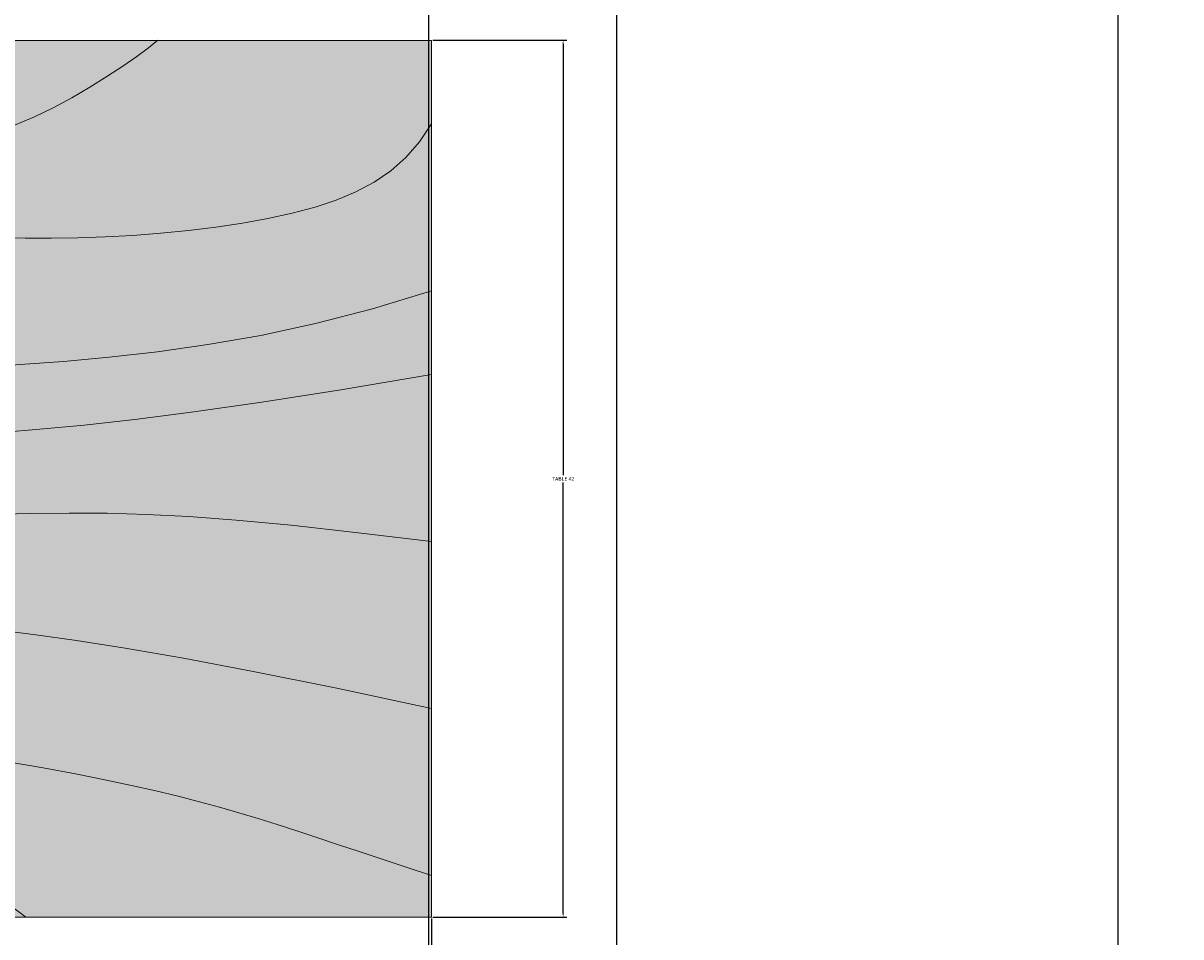
# Model space of a CAD drawing. Units: inches. Extents: x 1567 to 1964, y 1813 to 2447.
# Tile 11 of 28: x 1683 to 1738, y 2180 to 2224. Entities that reach past the tile are written whole.
import ezdxf

# ---------------------------------------------------------------- set-up
doc = ezdxf.new("R2010")
doc.units = ezdxf.units.IN
doc.layers.add('A-ANNO-DIMS', color=2, linetype='Continuous', lineweight=18)
doc.layers.add('A-FURN', color=8, linetype='Continuous', lineweight=18)
doc.layers.add('A-FURN-PATT', color=252, linetype='Continuous', lineweight=13, true_color=0x939598)
doc.styles.get("Standard").update_dxf_attribs({"font": 'arial.ttf'})
doc.dimstyles.get("Standard").update_dxf_attribs({"dimtxt": 0.18, "dimasz": 0.18, "dimexe": 0.18, "dimexo": 0.0625, "dimgap": 0.09, "dimtad": 0, "dimtih": 1, "dimtoh": 1, "dimdec": 4, "dimzin": 0, "dimdsep": 46, "dimtxsty": 'Standard', "dimcen": 0.09, "dimadec": 0, "dimazin": 0, "dimtfac": 1, "dimtdec": 4, "dimtofl": 0, "dimtmove": 0, "dimatfit": 3, "dimfxl": 1, "dimtolj": 1, "dimtzin": 0, "dimarcsym": 0})

# ---------------------------------------------------------------- blocks, each defined once
blk = doc.blocks.new('Table - Square Woodgrain 42 x 42 in.')
blk.add_line((0, -42), (42, -42))
for points in [[(0, -4), (1.704, -4.2172), (3.2358, -4.4188), (4.615, -4.604), (5.8615, -4.7721), (6.9951, -4.9224), (8.0357, -5.0541), (9.0031, -5.1667), (9.9171, -5.2594), (10.7951, -5.3316), (11.6445, -5.3836), (12.4702, -5.4157), (13.277, -5.4283), (14.0698, -5.4217), (14.8535, -5.3964), (15.6331, -5.3526), (16.4133, -5.2908), (17.1986, -5.2103), (17.9913, -5.1062), (18.793, -4.9727), (19.6056, -4.8038), (20.4307, -4.5937), (21.2701, -4.3365), (22.1256, -4.0262), (22.9989, -3.6571), (23.888, -3.2272), (24.7756, -2.7516), (25.6408, -2.2491), (26.4624, -1.7387), (27.2195, -1.2395), (27.891, -0.7703), (28.456, -0.3501), (28.8934, 0.002)], [(0, -42), (0, 0), (42, 0), (42, -42)], [(0, -8), (1.8203, -8.1001), (3.6741, -8.2149), (5.5411, -8.3408), (7.4011, -8.4741), (9.2339, -8.6112), (11.0193, -8.7484), (12.7371, -8.8821), (14.3671, -9.0086), (15.8954, -9.1246), (17.3337, -9.2278), (18.6997, -9.3159), (20.0116, -9.387), (21.2871, -9.4389), (22.5442, -9.4696), (23.8008, -9.477), (25.0749, -9.459), (26.3791, -9.4137), (27.7049, -9.3403), (29.0383, -9.2382), (30.3655, -9.1068), (31.6728, -8.9455), (32.9461, -8.7535), (34.1717, -8.5304), (35.3358, -8.2756), (36.4268, -7.9863), (37.443, -7.6521), (38.3849, -7.2603), (39.253, -6.7986), (40.048, -6.2542), (40.7705, -5.6147), (41.421, -4.8674), (42, -4)], [(42, -12), (39.1784, -12.8621), (36.4519, -13.5654), (33.8246, -14.1294), (31.3004, -14.5731), (28.8832, -14.9161), (26.577, -15.1775), (24.3858, -15.3768), (22.3136, -15.5332), (20.3622, -15.6632), (18.5254, -15.7718), (16.7947, -15.8612), (15.1618, -15.9338), (13.6183, -15.9916), (12.1558, -16.0369), (10.7659, -16.0718), (9.4403, -16.0987), (8.1703, -16.1191), (6.9461, -16.1325), (5.7577, -16.1377), (4.595, -16.1335), (3.4479, -16.1188), (2.3064, -16.0924), (1.1604, -16.0532), (0, -16)], [(42, -16), (37.6529, -16.7365), (33.8802, -17.329), (30.6179, -17.7961), (27.8015, -18.1561), (25.3668, -18.4275), (23.2497, -18.6288), (21.3859, -18.7785), (19.7111, -18.8949), (18.1693, -18.9939), (16.7375, -19.0795), (15.401, -19.1534), (14.1449, -19.217), (12.9544, -19.2717), (11.8148, -19.3191), (10.7113, -19.3606), (9.6291, -19.3976), (8.5534, -19.4323), (7.47, -19.4689), (6.3643, -19.5122), (5.222, -19.5672), (4.0288, -19.6386), (2.7703, -19.7313), (1.4321, -19.8501), (0, -20)], [(0, -24), (3.9243, -23.6805), (7.4766, -23.4138), (10.6891, -23.1954), (13.5943, -23.0205), (16.2247, -22.8847), (18.6125, -22.7832), (20.7903, -22.7116), (22.7903, -22.6651), (24.6563, -22.642), (26.4764, -22.6507), (28.35, -22.7024), (30.3766, -22.8084), (32.6555, -22.98), (35.2861, -23.2283), (38.3678, -23.5645), (42, -24)], [(42, -32), (37.392, -31.017), (33.4585, -30.2231), (30.1291, -29.5949), (27.3334, -29.109), (25.0009, -28.742), (23.0612, -28.4707), (21.4439, -28.2716), (20.0786, -28.1215), (18.8998, -28.0002), (17.8609, -27.9014), (16.9206, -27.8219), (16.0371, -27.7588), (15.1691, -27.709), (14.2748, -27.6693), (13.3128, -27.6368), (12.2415, -27.6083), (11.0295, -27.5824), (9.6867, -27.5643), (8.233, -27.5608), (6.6884, -27.5787), (5.0728, -27.6248), (3.4062, -27.7058), (1.7086, -27.8286), (0, -28)], [(0, -32), (5.4026, -32.5358), (9.9494, -33.019), (13.7424, -33.4553), (16.8834, -33.8505), (19.4743, -34.2106), (21.6171, -34.5413), (23.4136, -34.8486), (24.9657, -35.1382), (26.3614, -35.4156), (27.6332, -35.6841), (28.7995, -35.9467), (29.8788, -36.2064), (30.8897, -36.4661), (31.8507, -36.7288), (32.7802, -36.9973), (33.6968, -37.2747), (34.6175, -37.5635), (35.5531, -37.8651), (36.5128, -38.1805), (37.506, -38.5108), (38.5421, -38.8568), (39.6302, -39.2197), (40.7797, -39.6004), (42, -40)], [(0, -36), (3.0098, -36.2857), (5.5354, -36.5643), (7.6368, -36.8359), (9.374, -37.1009), (10.807, -37.3597), (11.9957, -37.6126), (13.0002, -37.8599), (13.8804, -38.102), (14.6874, -38.3393), (15.4365, -38.5729), (16.1338, -38.8041), (16.7858, -39.0341), (17.3987, -39.264), (17.9787, -39.4952), (18.5322, -39.7288), (19.0655, -39.9662), (19.5832, -40.2081), (20.0842, -40.4544), (20.5657, -40.7046), (21.0249, -40.9581), (21.459, -41.2144), (21.8653, -41.4731), (22.2409, -41.7335), (22.5831, -41.9951)]]:
    blk.add_lwpolyline(points)
blk = doc.blocks.new('*D25')
at = {"layer": 'A-ANNO-DIMS', "color": 0, "lineweight": -2, "transparency": 16777216}
for p, q in [((1702.624, 2222.808), (1709.041, 2222.808)), ((1708.861, 2222.628), (1708.861, 2201.987)), ((1708.861, 2180.986), (1708.861, 2201.626)), ((1702.624, 2180.806), (1709.041, 2180.806))]:
    blk.add_line(p, q, dxfattribs=at)
at = {"layer": 'A-ANNO-DIMS', "color": 0, "transparency": 16777216}
for points in [[(1708.831, 2222.628), (1708.891, 2222.628), (1708.861, 2222.808)], [(1708.831, 2180.986), (1708.891, 2180.986), (1708.861, 2180.806)]]:
    blk.add_solid(points, dxfattribs=at)
at = {"layer": 'Defpoints', "color": 0, "transparency": 16777216}
for p in [(1702.561, 2222.808), (1708.861, 2222.808), (1702.561, 2180.806)]:
    blk.add_point(p, dxfattribs=at)
at = {"layer": 'A-ANNO-DIMS', "color": 0, "transparency": 16777216, "insert": (1708.861, 2201.807), "char_height": 0.18, "attachment_point": 5}
blk.add_mtext('\\A1;TABLE 42', dxfattribs=at)
blk = doc.blocks.new('*D26')
at = {"layer": 'A-ANNO-DIMS', "color": 0, "lineweight": -2, "transparency": 16777216}
for p, q in [((1660.561, 2180.743), (1660.561, 2174.325)), ((1702.561, 2180.743), (1702.561, 2174.325)), ((1660.741, 2174.505), (1681.339, 2174.505)), ((1702.381, 2174.505), (1681.783, 2174.505))]:
    blk.add_line(p, q, dxfattribs=at)
at = {"layer": 'A-ANNO-DIMS', "color": 0, "transparency": 16777216}
for points in [[(1660.741, 2174.535), (1660.741, 2174.475), (1660.561, 2174.505)], [(1702.381, 2174.535), (1702.381, 2174.475), (1702.561, 2174.505)]]:
    blk.add_solid(points, dxfattribs=at)
at = {"layer": 'Defpoints', "color": 0, "transparency": 16777216}
for p in [(1660.561, 2180.806), (1702.561, 2180.806), (1702.561, 2174.505)]:
    blk.add_point(p, dxfattribs=at)
at = {"layer": 'A-ANNO-DIMS', "color": 0, "transparency": 16777216, "insert": (1681.561, 2174.505), "char_height": 0.18, "attachment_point": 5}
blk.add_mtext('\\A1;42', dxfattribs=at)
blk = doc.blocks.new('*D54')
at = {"layer": 'A-ANNO-DIMS', "color": 0, "lineweight": -2, "transparency": 16777216}
for p, q in [((1711.43, 1964.352), (1711.43, 2447.12)), ((1711.61, 2446.94), (1753.211, 2446.94)), ((1795.25, 2446.94), (1753.648, 2446.94)), ((1795.43, 1964.352), (1795.43, 2447.12))]:
    blk.add_line(p, q, dxfattribs=at)
at = {"layer": 'A-ANNO-DIMS', "color": 0, "transparency": 16777216}
for points in [[(1711.61, 2446.97), (1711.61, 2446.91), (1711.43, 2446.94)], [(1795.25, 2446.97), (1795.25, 2446.91), (1795.43, 2446.94)]]:
    blk.add_solid(points, dxfattribs=at)
at = {"layer": 'Defpoints', "color": 0, "transparency": 16777216}
for p in [(1795.43, 2446.94), (1711.43, 1964.29), (1795.43, 1964.29)]:
    blk.add_point(p, dxfattribs=at)
at = {"layer": 'A-ANNO-DIMS', "color": 0, "transparency": 16777216, "insert": (1753.43, 2446.94), "char_height": 0.18, "attachment_point": 5}
blk.add_mtext('\\A1;84', dxfattribs=at)
blk = doc.blocks.new('*D60')
at = {"layer": 'A-ANNO-DIMS', "color": 0, "lineweight": -2, "transparency": 16777216}
for p, q in [((1660.43, 2063.352), (1660.43, 2447.12)), ((1660.61, 2446.94), (1681.208, 2446.94)), ((1702.25, 2446.94), (1681.651, 2446.94)), ((1702.43, 2063.352), (1702.43, 2447.12))]:
    blk.add_line(p, q, dxfattribs=at)
at = {"layer": 'A-ANNO-DIMS', "color": 0, "transparency": 16777216}
for points in [[(1660.61, 2446.97), (1660.61, 2446.91), (1660.43, 2446.94)], [(1702.25, 2446.97), (1702.25, 2446.91), (1702.43, 2446.94)]]:
    blk.add_solid(points, dxfattribs=at)
at = {"layer": 'Defpoints', "color": 0, "transparency": 16777216}
for p in [(1660.43, 2446.94), (1660.43, 2063.29), (1702.43, 2063.29)]:
    blk.add_point(p, dxfattribs=at)
at = {"layer": 'A-ANNO-DIMS', "color": 0, "transparency": 16777216, "insert": (1681.43, 2446.94), "char_height": 0.18, "attachment_point": 5}
blk.add_mtext('\\A1;42', dxfattribs=at)
blk = doc.blocks.new('*D63')
at = {"layer": 'A-ANNO-DIMS', "color": 0, "lineweight": -2, "transparency": 16777216}
for p, q in [((1735.43, 1988.352), (1735.43, 2447.12)), ((1735.61, 2446.94), (1753.211, 2446.94)), ((1771.25, 2446.94), (1753.648, 2446.94)), ((1771.43, 1988.352), (1771.43, 2447.12))]:
    blk.add_line(p, q, dxfattribs=at)
at = {"layer": 'A-ANNO-DIMS', "color": 0, "transparency": 16777216}
for points in [[(1735.61, 2446.97), (1735.61, 2446.91), (1735.43, 2446.94)], [(1771.25, 2446.97), (1771.25, 2446.91), (1771.43, 2446.94)]]:
    blk.add_solid(points, dxfattribs=at)
at = {"layer": 'Defpoints', "color": 0, "transparency": 16777216}
for p in [(1771.43, 2446.94), (1735.43, 1988.29), (1771.43, 1988.29)]:
    blk.add_point(p, dxfattribs=at)
at = {"layer": 'A-ANNO-DIMS', "color": 0, "transparency": 16777216, "insert": (1753.43, 2446.94), "char_height": 0.18, "attachment_point": 5}
blk.add_mtext('\\A1;36', dxfattribs=at)
blk = doc.blocks.new('*D64')
at = {"layer": 'A-ANNO-DIMS', "color": 0, "lineweight": -2, "transparency": 16777216}
for p, q in [((1711.43, 2055.852), (1711.43, 2447.12)), ((1711.61, 2446.94), (1723.209, 2446.94)), ((1735.25, 2446.94), (1723.65, 2446.94)), ((1735.43, 2055.852), (1735.43, 2447.12))]:
    blk.add_line(p, q, dxfattribs=at)
at = {"layer": 'A-ANNO-DIMS', "color": 0, "transparency": 16777216}
for points in [[(1711.61, 2446.97), (1711.61, 2446.91), (1711.43, 2446.94)], [(1735.25, 2446.97), (1735.25, 2446.91), (1735.43, 2446.94)]]:
    blk.add_solid(points, dxfattribs=at)
at = {"layer": 'Defpoints', "color": 0, "transparency": 16777216}
for p in [(1735.43, 2446.94), (1711.43, 2055.79), (1735.43, 2055.79)]:
    blk.add_point(p, dxfattribs=at)
at = {"layer": 'A-ANNO-DIMS', "color": 0, "transparency": 16777216, "insert": (1723.43, 2446.94), "char_height": 0.18, "attachment_point": 5}
blk.add_mtext('\\A1;24', dxfattribs=at)

msp = doc.modelspace()

# ---------------------------------------------------------------- hatches: boundary and pattern name
at = {"layer": 'A-FURN-PATT'}
h = msp.add_hatch(color=256, dxfattribs=at)
h.dxf.hatch_style = 1
h.paths.add_polyline_path([(1697.3402, 2374.8316), (1682.1402, 2374.8316), (1682.1402, 2387.6316), (1637.3402, 2387.6316), (1637.3402, 2324.4315), (1697.3402, 2324.4315)])
h.paths.add_polyline_path([(1891.1093, 2375.8204), (1875.9094, 2375.8204), (1875.9094, 2388.6204), (1831.1094, 2388.6204), (1831.1094, 2325.4204), (1891.1093, 2325.4204)])
h.paths.add_polyline_path([(1702.5611, 2206.8057), (1702.5611, 2210.8057), (1699.7395, 2209.9436), (1697.013, 2209.2403), (1694.3857, 2208.6763), (1691.8615, 2208.2326), (1689.4443, 2207.8896), (1687.1381, 2207.6282), (1684.9469, 2207.4289), (1682.8747, 2207.2725), (1680.9233, 2207.1425), (1679.0865, 2207.0339), (1677.3558, 2206.9445), (1675.7229, 2206.8719), (1674.1794, 2206.8141), (1672.7169, 2206.7688), (1671.327, 2206.7339), (1670.0014, 2206.707), (1668.7314, 2206.6866), (1667.5072, 2206.6732), (1666.3188, 2206.668), (1665.1561, 2206.6722), (1664.009, 2206.6869), (1662.8675, 2206.7133), (1661.7215, 2206.7525), (1660.5611, 2206.8057), (1660.5611, 2202.8057), (1661.9932, 2202.9556), (1663.3314, 2203.0744), (1664.5899, 2203.1671), (1665.7831, 2203.2385), (1666.9254, 2203.2935), (1668.0311, 2203.3368), (1669.1145, 2203.3734), (1670.1902, 2203.4081), (1671.2724, 2203.4451), (1672.3759, 2203.4866), (1673.5155, 2203.534), (1674.706, 2203.5887), (1675.9621, 2203.6523), (1677.2986, 2203.7262), (1678.7304, 2203.8118), (1680.2722, 2203.9108), (1681.947, 2204.0272), (1683.8108, 2204.1769), (1685.9279, 2204.3782), (1688.3626, 2204.6496), (1691.179, 2205.0096), (1694.4413, 2205.4767), (1698.214, 2206.0692)])
h.paths.add_polyline_path([(1702.5611, 2218.8057), (1701.9821, 2217.9383), (1701.3316, 2217.191), (1700.6091, 2216.5515), (1699.8141, 2216.0071), (1698.946, 2215.5454), (1698.0041, 2215.1536), (1696.9879, 2214.8194), (1695.8969, 2214.5301), (1694.7328, 2214.2753), (1693.5072, 2214.0522), (1692.2339, 2213.8602), (1690.9266, 2213.6989), (1689.5994, 2213.5675), (1688.266, 2213.4654), (1686.9402, 2213.392), (1685.636, 2213.3467), (1684.3619, 2213.3287), (1683.1053, 2213.3361), (1681.8482, 2213.3668), (1680.5727, 2213.4187), (1679.2608, 2213.4898), (1677.8948, 2213.5779), (1676.4565, 2213.6811), (1674.9282, 2213.7971), (1673.2982, 2213.9236), (1671.5804, 2214.0573), (1669.795, 2214.1945), (1667.9622, 2214.3316), (1666.1022, 2214.4649), (1664.2352, 2214.5908), (1662.3814, 2214.7056), (1660.5611, 2214.8057), (1660.5611, 2206.8057), (1661.7215, 2206.7525), (1662.8675, 2206.7133), (1664.009, 2206.6869), (1665.1561, 2206.6722), (1666.3188, 2206.668), (1667.5072, 2206.6732), (1668.7314, 2206.6866), (1670.0014, 2206.707), (1671.327, 2206.7339), (1672.7169, 2206.7688), (1674.1794, 2206.8141), (1675.7229, 2206.8719), (1677.3558, 2206.9445), (1679.0865, 2207.0339), (1680.9233, 2207.1425), (1682.8747, 2207.2725), (1684.9469, 2207.4289), (1687.1381, 2207.6282), (1689.4443, 2207.8896), (1691.8615, 2208.2326), (1694.3857, 2208.6763), (1697.013, 2209.2403), (1699.7395, 2209.9436), (1702.5611, 2210.8057)])
h.paths.add_polyline_path([(1700.6091, 2216.5515), (1701.3316, 2217.191), (1701.9821, 2217.9383), (1702.5611, 2218.8057), (1702.5611, 2222.8057), (1689.452, 2222.8057), (1689.0171, 2222.4556), (1688.4521, 2222.0354), (1687.7806, 2221.5662), (1687.0235, 2221.067), (1686.2019, 2220.5566), (1685.3367, 2220.0541), (1684.4491, 2219.5785), (1683.56, 2219.1486), (1682.6867, 2218.7795), (1681.8312, 2218.4692), (1680.9918, 2218.212), (1680.1667, 2218.0019), (1679.3541, 2217.833), (1678.5524, 2217.6995), (1677.7597, 2217.5954), (1676.9744, 2217.5149), (1676.1942, 2217.4531), (1675.4146, 2217.4093), (1674.6309, 2217.384), (1673.8381, 2217.3774), (1673.0313, 2217.39), (1672.2056, 2217.4221), (1671.3562, 2217.4741), (1670.4782, 2217.5463), (1669.5642, 2217.639), (1668.5968, 2217.7516), (1667.5562, 2217.8833), (1666.4226, 2218.0336), (1665.1761, 2218.2017), (1663.7969, 2218.3869), (1662.2651, 2218.5885), (1660.5611, 2218.8057), (1660.5611, 2214.8057), (1662.3814, 2214.7056), (1664.2352, 2214.5908), (1666.1022, 2214.4649), (1667.9622, 2214.3316), (1669.795, 2214.1945), (1671.5804, 2214.0573), (1673.2982, 2213.9236), (1674.9282, 2213.7971), (1676.4565, 2213.6811), (1677.8948, 2213.5779), (1679.2608, 2213.4898), (1680.5727, 2213.4187), (1681.8482, 2213.3668), (1683.1053, 2213.3361), (1684.3619, 2213.3287), (1685.636, 2213.3467), (1686.9402, 2213.392), (1688.266, 2213.4654), (1689.5994, 2213.5675), (1690.9266, 2213.6989), (1692.2339, 2213.8602), (1693.5072, 2214.0522), (1694.7328, 2214.2753), (1695.8969, 2214.5301), (1696.9879, 2214.8194), (1698.0041, 2215.1536), (1698.946, 2215.5454), (1699.8141, 2216.0071)])
h.paths.add_polyline_path([(1687.0235, 2221.067), (1687.7806, 2221.5662), (1688.4521, 2222.0354), (1689.0171, 2222.4556), (1689.452, 2222.8057), (1660.5611, 2222.8057), (1660.5611, 2218.8057), (1662.2651, 2218.5885), (1663.7969, 2218.3869), (1665.1761, 2218.2017), (1666.4226, 2218.0336), (1667.5562, 2217.8833), (1668.5968, 2217.7516), (1669.5642, 2217.639), (1670.4782, 2217.5463), (1671.3562, 2217.4741), (1672.2056, 2217.4221), (1673.0313, 2217.39), (1673.8381, 2217.3774), (1674.6309, 2217.384), (1675.4146, 2217.4093), (1676.1942, 2217.4531), (1676.9744, 2217.5149), (1677.7597, 2217.5954), (1678.5524, 2217.6995), (1679.3541, 2217.833), (1680.1667, 2218.0019), (1680.9918, 2218.212), (1681.8312, 2218.4692), (1682.6867, 2218.7795), (1683.56, 2219.1486), (1684.4491, 2219.5785), (1685.3367, 2220.0541), (1686.2019, 2220.5566)], flags=17)
h.paths.add_polyline_path([(1702.5611, 2198.8057), (1698.9289, 2199.2412), (1695.8472, 2199.5774), (1693.2166, 2199.8257), (1690.9377, 2199.9973), (1688.9111, 2200.1033), (1687.0375, 2200.155), (1685.2174, 2200.1637), (1683.3514, 2200.1406), (1681.3514, 2200.0941), (1679.1736, 2200.0225), (1676.7858, 2199.921), (1674.1554, 2199.7852), (1671.2502, 2199.6103), (1668.0377, 2199.3919), (1664.4854, 2199.1252), (1660.5611, 2198.8057), (1660.5611, 2194.8057), (1662.2697, 2194.9771), (1663.9673, 2195.0999), (1665.6339, 2195.1809), (1667.2495, 2195.227), (1668.7941, 2195.2449), (1670.2478, 2195.2414), (1671.5906, 2195.2233), (1672.8026, 2195.1974), (1673.8739, 2195.1689), (1674.8359, 2195.1364), (1675.7302, 2195.0967), (1676.5982, 2195.0469), (1677.4817, 2194.9838), (1678.422, 2194.9043), (1679.4609, 2194.8055), (1680.6397, 2194.6842), (1682.005, 2194.5341), (1683.6223, 2194.335), (1685.562, 2194.0637), (1687.8945, 2193.6967), (1690.6902, 2193.2108), (1694.0196, 2192.5826), (1697.9531, 2191.7887), (1702.5611, 2190.8057)])
h.paths.add_polyline_path([(1702.5611, 2206.8057), (1698.214, 2206.0692), (1694.4413, 2205.4767), (1691.179, 2205.0096), (1688.3626, 2204.6496), (1685.9279, 2204.3782), (1683.8108, 2204.1769), (1681.947, 2204.0272), (1680.2722, 2203.9108), (1678.7304, 2203.8118), (1677.2986, 2203.7262), (1675.9621, 2203.6523), (1674.706, 2203.5887), (1673.5155, 2203.534), (1672.3759, 2203.4866), (1671.2724, 2203.4451), (1670.1902, 2203.4081), (1669.1145, 2203.3734), (1668.0311, 2203.3368), (1666.9254, 2203.2935), (1665.7831, 2203.2385), (1664.5899, 2203.1671), (1663.3314, 2203.0744), (1661.9932, 2202.9556), (1660.5611, 2202.8057), (1660.5611, 2198.8057), (1664.4854, 2199.1252), (1668.0377, 2199.3919), (1671.2502, 2199.6103), (1674.1554, 2199.7852), (1676.7858, 2199.921), (1679.1736, 2200.0225), (1681.3514, 2200.0941), (1683.3514, 2200.1406), (1685.2174, 2200.1637), (1687.0375, 2200.155), (1688.9111, 2200.1033), (1690.9377, 2199.9973), (1693.2166, 2199.8257), (1695.8472, 2199.5774), (1698.9289, 2199.2412), (1702.5611, 2198.8057)])
h.paths.add_polyline_path([(1702.5611, 2190.8057), (1697.9531, 2191.7887), (1694.0196, 2192.5826), (1690.6902, 2193.2108), (1687.8945, 2193.6967), (1685.562, 2194.0637), (1683.6223, 2194.335), (1682.005, 2194.5341), (1680.6397, 2194.6842), (1679.4609, 2194.8055), (1678.422, 2194.9043), (1677.4817, 2194.9838), (1676.5982, 2195.0469), (1675.7302, 2195.0967), (1674.8359, 2195.1364), (1673.8739, 2195.1689), (1672.8026, 2195.1974), (1671.5906, 2195.2233), (1670.2478, 2195.2414), (1668.7941, 2195.2449), (1667.2495, 2195.227), (1665.6339, 2195.1809), (1663.9673, 2195.0999), (1662.2697, 2194.9771), (1660.5611, 2194.8057), (1660.5611, 2190.8057), (1665.9637, 2190.2699), (1670.5105, 2189.7867), (1674.3035, 2189.3504), (1677.4445, 2188.9552), (1680.0354, 2188.5951), (1682.1782, 2188.2644), (1683.9747, 2187.9571), (1685.5268, 2187.6675), (1686.9225, 2187.3901), (1688.1943, 2187.1216), (1689.3606, 2186.859), (1690.4399, 2186.5993), (1691.4508, 2186.3396), (1692.4118, 2186.0769), (1693.3413, 2185.8084), (1694.2579, 2185.531), (1695.1786, 2185.2422), (1696.1142, 2184.9406), (1697.0739, 2184.6252), (1698.0671, 2184.2949), (1699.1032, 2183.9489), (1700.1913, 2183.586), (1701.3408, 2183.2053), (1702.5611, 2182.8057)])
h.paths.add_polyline_path([(1702.5611, 2182.8057), (1701.3408, 2183.2053), (1700.1913, 2183.586), (1699.1032, 2183.9489), (1698.0671, 2184.2949), (1697.0739, 2184.6252), (1696.1142, 2184.9406), (1695.1786, 2185.2422), (1694.2579, 2185.531), (1693.3413, 2185.8084), (1692.4118, 2186.0769), (1691.4508, 2186.3396), (1690.4399, 2186.5993), (1689.3606, 2186.859), (1688.1943, 2187.1216), (1686.9225, 2187.3901), (1685.5268, 2187.6675), (1683.9747, 2187.9571), (1682.1782, 2188.2644), (1680.0354, 2188.5951), (1677.4445, 2188.9552), (1674.3035, 2189.3504), (1670.5105, 2189.7867), (1665.9637, 2190.2699), (1660.5611, 2190.8057), (1660.5611, 2186.8057), (1663.5709, 2186.52), (1666.0965, 2186.2414), (1668.1979, 2185.9698), (1669.9351, 2185.7048), (1671.3681, 2185.446), (1672.5568, 2185.1931), (1673.5613, 2184.9458), (1674.4415, 2184.7037), (1675.2485, 2184.4664), (1675.9976, 2184.2328), (1677.0295, 2183.8907), (1678.2492, 2183.4332), (1679.354, 2182.9669), (1680.4123, 2182.4724), (1681.3757, 2181.9718), (1682.2435, 2181.4594), (1683.1864, 2180.8057), (1702.5611, 2180.8057)])
h.paths.add_polyline_path([(1677.3469, 2183.7716), (1676.6949, 2184.0016), (1675.9976, 2184.2328), (1675.2485, 2184.4664), (1674.4415, 2184.7037), (1673.5613, 2184.9458), (1672.5568, 2185.1931), (1671.3681, 2185.446), (1669.9351, 2185.7048), (1668.1979, 2185.9698), (1666.0965, 2186.2414), (1663.5709, 2186.52), (1660.5611, 2186.8057), (1660.5611, 2180.8057), (1683.1506, 2180.8057), (1682.802, 2181.0722), (1682.4264, 2181.3326), (1682.0201, 2181.5913), (1681.586, 2181.8476), (1681.1268, 2182.1011), (1680.6453, 2182.3513), (1680.1443, 2182.5976), (1679.6266, 2182.8395), (1679.0933, 2183.0769), (1678.5398, 2183.3105), (1677.9598, 2183.5417)], flags=17)
h.paths.add_polyline_path([(1824.4511, 2199.9016), (1824.089, 2199.9302), (1824.0595, 2199.9372), (1824.0397, 2199.9406), (1823.5413, 2200.0576), (1823.4095, 2200.0864), (1823.0664, 2200.1559), (1822.6419, 2200.2361), (1822.1519, 2200.3222), (1821.6126, 2200.4093), (1821.0401, 2200.4925), (1820.4505, 2200.5669), (1819.8599, 2200.6276), (1819.2845, 2200.6697), (1818.7366, 2200.6896), (1818.2141, 2200.688), (1817.7112, 2200.6668), (1817.222, 2200.6281), (1816.7405, 2200.5737), (1816.261, 2200.5057), (1815.7776, 2200.4259), (1815.2845, 2200.3364), (1814.3007, 2200.149), (1813.3315, 2199.9765), (1812.406, 2199.8514), (1811.6868, 2199.7739), (1810.8992, 2199.7121), (1810.0345, 2199.6697), (1809.0854, 2199.6497), (1808.0514, 2199.6502), (1806.9334, 2199.6683), (1805.7324, 2199.701), (1804.4493, 2199.7454), (1803.0852, 2199.7986), (1801.641, 2199.8577), (1800.1178, 2199.9197), (1798.5134, 2199.9818), (1796.8144, 2200.0415), (1795.004, 2200.0962), (1793.0657, 2200.1437), (1790.9828, 2200.1814), (1788.7389, 2200.2068), (1786.3171, 2200.2177), (1783.7011, 2200.2114), (1780.8715, 2200.185), (1777.7988, 2200.1326), (1774.4506, 2200.0481), (1770.7948, 2199.9249), (1766.7992, 2199.7569), (1762.4316, 2199.5376), (1757.6596, 2199.2606), (1752.4511, 2198.9197), (1752.4511, 2193.4197), (1761.2668, 2193.6071), (1768.3671, 2193.7934), (1773.9821, 2193.9778), (1778.3417, 2194.1593), (1781.6759, 2194.3369), (1784.2148, 2194.5096), (1786.1882, 2194.6764), (1787.8261, 2194.8364), (1789.3219, 2194.9887), (1790.7226, 2195.1333), (1792.0383, 2195.27), (1793.2792, 2195.3989), (1794.4557, 2195.52), (1795.5781, 2195.6333), (1796.6564, 2195.7387), (1797.7011, 2195.8364), (1798.7216, 2195.9259), (1799.7245, 2196.0057), (1800.7158, 2196.0737), (1801.7011, 2196.1281), (1802.6865, 2196.1668), (1803.6777, 2196.188), (1804.6806, 2196.1896), (1805.7011, 2196.1697), (1806.7423, 2196.1273), (1807.7962, 2196.0643), (1808.852, 2195.9837), (1809.899, 2195.8885), (1810.9265, 2195.7815), (1811.9238, 2195.6658), (1812.88, 2195.5442), (1813.7845, 2195.4197), (1814.6296, 2195.2948), (1815.4205, 2195.1704), (1816.1656, 2195.0469), (1816.873, 2194.9249), (1817.5511, 2194.8049), (1818.2083, 2194.6873), (1818.8527, 2194.5726), (1819.4928, 2194.4614), (1820.1348, 2194.3554), (1820.7773, 2194.2615), (1821.4169, 2194.1882), (1822.0501, 2194.1437), (1822.6735, 2194.1363), (1823.2838, 2194.1743), (1823.8775, 2194.266), (1824.4511, 2194.4197)])
h.paths.add_polyline_path([(1821.4716, 2190.5098), (1820.4303, 2190.5708), (1819.3811, 2190.6415), (1818.3339, 2190.7186), (1817.2985, 2190.7986), (1816.2845, 2190.8781), (1815.2976, 2190.9542), (1814.3274, 2191.0259), (1813.3592, 2191.0927), (1812.3782, 2191.1541), (1811.3699, 2191.2097), (1810.3196, 2191.2589), (1809.2127, 2191.3013), (1808.0345, 2191.3364), (1806.7708, 2191.3634), (1805.4094, 2191.3807), (1803.9387, 2191.3862), (1802.3469, 2191.3781), (1800.6223, 2191.3543), (1798.7532, 2191.313), (1796.7278, 2191.2521), (1794.5344, 2191.1697), (1792.128, 2191.0648), (1789.33, 2190.9393), (1785.9285, 2190.7962), (1781.7115, 2190.6385), (1776.4672, 2190.469), (1769.9836, 2190.2908), (1762.0489, 2190.1067), (1752.4511, 2189.9197), (1752.4511, 2185.4197), (1758.363, 2185.5846), (1763.4179, 2185.7075), (1767.7199, 2185.7933), (1771.373, 2185.8468), (1774.4811, 2185.873), (1777.1484, 2185.8768), (1779.4787, 2185.8629), (1781.5761, 2185.8364), (1783.5287, 2185.8014), (1785.3606, 2185.7596), (1787.0802, 2185.7119), (1788.6959, 2185.6593), (1790.2158, 2185.6028), (1791.6484, 2185.5434), (1793.0018, 2185.4821), (1794.2844, 2185.4197), (1795.5065, 2185.3576), (1796.6861, 2185.298), (1797.8433, 2185.2432), (1798.998, 2185.1958), (1800.1703, 2185.1581), (1801.3801, 2185.1326), (1802.6476, 2185.1218), (1803.9928, 2185.1281), (1805.4444, 2185.1555), (1807.0663, 2185.2147), (1808.9315, 2185.3178), (1811.1126, 2185.477), (1813.6823, 2185.7046), (1816.7135, 2186.0128), (1820.2788, 2186.4138), (1824.4511, 2186.9197), (1824.4511, 2190.4197), (1823.4918, 2190.4309), (1822.4954, 2190.4621)])
h.paths.add_polyline_path([(1797.3762, 2216.0584), (1797.6199, 2216.2267), (1797.9558, 2216.3355), (1798.3017, 2216.3703), (1798.5761, 2216.3781), (1798.8974, 2216.3703), (1799.2714, 2216.3468), (1799.704, 2216.3078), (1800.2011, 2216.2531), (1800.7695, 2216.1829), (1801.4205, 2216.0981), (1802.1662, 2215.9996), (1803.0188, 2215.8885), (1803.9906, 2215.7656), (1805.0937, 2215.632), (1806.3404, 2215.4886), (1807.7428, 2215.3364), (1809.3101, 2215.1764), (1811.039, 2215.0096), (1812.9232, 2214.8369), (1814.9563, 2214.6593), (1817.132, 2214.4778), (1819.444, 2214.2934), (1821.8858, 2214.1071), (1824.4511, 2213.9197), (1824.4511, 2217.9197), (1752.4511, 2217.9197), (1752.4511, 2214.9197), (1757.2739, 2214.8973), (1761.6432, 2214.8338), (1765.5973, 2214.7352), (1769.1751, 2214.6072), (1772.4149, 2214.4559), (1775.3554, 2214.2869), (1778.0352, 2214.1063), (1780.4928, 2213.9197), (1782.7607, 2213.7329), (1784.8476, 2213.5499), (1786.7557, 2213.3748), (1788.4876, 2213.2114), (1790.0456, 2213.0636), (1791.4322, 2212.9354), (1792.6499, 2212.8305), (1793.7011, 2212.7531), (1794.5904, 2212.7059), (1795.3313, 2212.688), (1795.9394, 2212.6974), (1796.4303, 2212.7322), (1796.8196, 2212.7905), (1797.123, 2212.8703), (1797.356, 2212.9695), (1797.5344, 2213.0864), (1797.6716, 2213.2187), (1797.7727, 2213.3637), (1797.8406, 2213.5185), (1797.8782, 2213.6801), (1797.8884, 2213.8457), (1797.8743, 2214.0122), (1797.8386, 2214.1767), (1797.7844, 2214.3364), (1797.7149, 2214.4889), (1797.6347, 2214.6346), (1797.5486, 2214.7744), (1797.3327, 2215.109), (1797.178, 2215.4303), (1797.1896, 2215.7939)])
h.paths.add_polyline_path([(1804.7872, 2210.6789), (1804.546, 2211.022), (1804.3512, 2211.3917), (1804.2466, 2211.7546), (1804.2574, 2212.0998), (1804.4058, 2212.4178), (1804.7068, 2212.7007), (1805.1359, 2212.9124), (1805.5279, 2212.9926), (1805.8136, 2213.0154), (1806.1178, 2213.0031), (1806.4405, 2212.9529), (1806.7929, 2212.867), (1807.1893, 2212.7489), (1807.6438, 2212.602), (1808.1706, 2212.4297), (1808.7838, 2212.2355), (1809.4976, 2212.0227), (1810.3261, 2211.7947), (1811.2868, 2211.5533), (1812.4101, 2211.2928), (1813.7297, 2211.0059), (1815.2793, 2210.6854), (1817.0925, 2210.3238), (1819.2031, 2209.9139), (1821.6447, 2209.4483), (1824.4511, 2208.9197), (1824.4511, 2213.9197), (1821.8858, 2214.1071), (1819.444, 2214.2934), (1817.132, 2214.4778), (1814.9563, 2214.6593), (1812.9232, 2214.8369), (1811.039, 2215.0096), (1809.3101, 2215.1764), (1807.7428, 2215.3364), (1806.3404, 2215.4886), (1805.0937, 2215.632), (1803.9906, 2215.7656), (1803.0188, 2215.8885), (1802.1662, 2215.9996), (1801.4205, 2216.0981), (1800.7695, 2216.1829), (1800.2011, 2216.2531), (1799.704, 2216.3078), (1799.2714, 2216.3468), (1798.8974, 2216.3703), (1798.5761, 2216.3781), (1798.3017, 2216.3703), (1798.0683, 2216.3468), (1797.87, 2216.3078), (1797.7011, 2216.2531), (1797.5566, 2216.1831), (1797.4355, 2216.0994), (1797.3378, 2216.004), (1797.2636, 2215.8989), (1797.2128, 2215.7859), (1797.1855, 2215.6671), (1797.1816, 2215.5444), (1797.2011, 2215.4197), (1797.2433, 2215.2946), (1797.304, 2215.1684), (1797.3783, 2215.0403), (1797.4615, 2214.9093), (1797.6718, 2214.5836), (1797.8218, 2214.2545), (1797.8933, 2213.9247), (1797.8728, 2213.5918), (1797.7366, 2213.2814), (1797.4586, 2213.0132), (1797.123, 2212.8703), (1796.8196, 2212.7905), (1796.4303, 2212.7322), (1795.9394, 2212.6974), (1795.3313, 2212.688), (1794.5904, 2212.7059), (1793.7011, 2212.7531), (1792.6499, 2212.8305), (1791.4322, 2212.9354), (1790.0456, 2213.0636), (1788.4876, 2213.2114), (1786.7557, 2213.3748), (1784.8476, 2213.5499), (1782.7607, 2213.7329), (1780.4928, 2213.9197), (1778.0352, 2214.1063), (1775.3554, 2214.2869), (1772.4149, 2214.4559), (1769.1751, 2214.6072), (1765.5973, 2214.7352), (1761.6432, 2214.8338), (1757.2739, 2214.8973), (1752.4511, 2214.9197), (1752.4511, 2209.9197), (1759.4745, 2210.0625), (1765.2786, 2210.1242), (1770.027, 2210.1175), (1773.8834, 2210.0551), (1777.0112, 2209.9498), (1779.5741, 2209.8143), (1781.7357, 2209.6611), (1783.6594, 2209.5031), (1785.4813, 2209.3506), (1787.2265, 2209.2049), (1788.8926, 2209.0651), (1790.4771, 2208.9301), (1791.9777, 2208.7991), (1793.3919, 2208.671), (1794.7171, 2208.5449), (1795.9511, 2208.4197), (1797.0922, 2208.2952), (1798.1425, 2208.1736), (1799.1049, 2208.0579), (1799.9823, 2207.951), (1800.7778, 2207.8558), (1801.4941, 2207.7752), (1802.1342, 2207.7122), (1802.7011, 2207.6697), (1803.1982, 2207.65), (1803.6308, 2207.6528), (1804.0048, 2207.6771), (1804.3261, 2207.7218), (1804.6005, 2207.7861), (1804.8339, 2207.869), (1805.0322, 2207.9694), (1805.2011, 2208.0864), (1805.3455, 2208.2189), (1805.4654, 2208.365), (1805.56, 2208.5229), (1805.6282, 2208.6906), (1805.6691, 2208.866), (1805.6816, 2209.0473), (1805.6648, 2209.2326), (1805.6178, 2209.4197), (1805.5406, 2209.6072), (1805.4381, 2209.7947), (1805.316, 2209.9822), (1805.1803, 2210.1697), (1805.0367, 2210.3572)])
h.paths.add_polyline_path([(1801.4941, 2207.7752), (1800.7778, 2207.8558), (1799.9823, 2207.951), (1799.1049, 2208.0579), (1798.1425, 2208.1736), (1797.0922, 2208.2952), (1795.9511, 2208.4197), (1794.7171, 2208.5449), (1793.3919, 2208.671), (1791.9777, 2208.7991), (1790.4771, 2208.9301), (1788.8926, 2209.0651), (1787.2265, 2209.2049), (1785.4813, 2209.3506), (1783.6594, 2209.5031), (1781.7357, 2209.6611), (1779.5741, 2209.8143), (1777.0112, 2209.9498), (1773.8834, 2210.0551), (1770.027, 2210.1175), (1765.2786, 2210.1242), (1759.4745, 2210.0625), (1752.4511, 2209.9197), (1752.4511, 2205.4197), (1757.7354, 2205.2545), (1762.3821, 2205.1294), (1766.4565, 2205.0374), (1770.024, 2204.9718), (1773.1502, 2204.9258), (1775.9003, 2204.8924), (1778.3399, 2204.8649), (1780.5344, 2204.8364), (1782.5421, 2204.8014), (1784.3925, 2204.7596), (1786.1082, 2204.7119), (1787.7115, 2204.6593), (1789.225, 2204.6028), (1790.6711, 2204.5434), (1792.0724, 2204.4821), (1793.4511, 2204.4197), (1794.8241, 2204.3576), (1796.1855, 2204.2973), (1797.5234, 2204.241), (1798.8261, 2204.1906), (1800.082, 2204.1479), (1801.2792, 2204.115), (1802.4062, 2204.0939), (1803.4511, 2204.0864), (1804.4051, 2204.0942), (1805.2701, 2204.1176), (1806.0512, 2204.1567), (1806.7532, 2204.2114), (1807.381, 2204.2817), (1807.9394, 2204.3676), (1808.4334, 2204.4692), (1808.8678, 2204.5864), (1809.248, 2204.7187), (1809.5813, 2204.8637), (1809.8756, 2205.0185), (1810.1386, 2205.1801), (1810.3782, 2205.3457), (1810.6022, 2205.5122), (1810.9725, 2205.7941), (1811.3803, 2206.072), (1811.739, 2206.2612), (1812.0032, 2206.3781), (1812.2869, 2206.4793), (1812.5931, 2206.563), (1812.9246, 2206.6271), (1813.2845, 2206.6697), (1813.6746, 2206.6894), (1814.0931, 2206.6867), (1814.5369, 2206.6624), (1815.0032, 2206.6176), (1815.489, 2206.5534), (1815.9915, 2206.4705), (1816.5076, 2206.3701), (1817.0345, 2206.2531), (1817.5753, 2206.1196), (1818.1582, 2205.9666), (1818.8172, 2205.7902), (1819.5865, 2205.5864), (1820.5004, 2205.3514), (1821.5931, 2205.0812), (1822.8986, 2204.7719), (1824.4511, 2204.4197), (1824.4511, 2208.9197), (1821.6447, 2209.4483), (1819.2031, 2209.9139), (1817.0925, 2210.3238), (1815.2793, 2210.6854), (1813.7297, 2211.0059), (1812.4101, 2211.2928), (1811.2868, 2211.5533), (1810.3261, 2211.7947), (1809.4976, 2212.0227), (1808.7838, 2212.2355), (1808.1706, 2212.4297), (1807.6438, 2212.602), (1807.1893, 2212.7489), (1806.7929, 2212.867), (1806.4405, 2212.9529), (1806.1178, 2213.0031), (1805.8136, 2213.0154), (1805.5279, 2212.9926), (1805.2638, 2212.9386), (1805.024, 2212.8572), (1804.8116, 2212.7524), (1804.6295, 2212.6281), (1804.4806, 2212.4881), (1804.3678, 2212.3364), (1804.2931, 2212.1764), (1804.2545, 2212.0096), (1804.2491, 2211.8369), (1804.274, 2211.6593), (1804.3263, 2211.4778), (1804.4029, 2211.2934), (1804.5011, 2211.1071), (1804.6178, 2210.9197), (1804.7496, 2210.7322), (1804.8912, 2210.5447), (1805.154, 2210.2061), (1805.3962, 2209.8715), (1805.5964, 2209.5053), (1805.688, 2209.1402), (1805.6629, 2208.7758), (1805.5257, 2208.4385), (1805.2839, 2208.1437), (1804.9434, 2207.9078), (1804.6005, 2207.7861), (1804.3261, 2207.7218), (1804.0048, 2207.6771), (1803.6308, 2207.6528), (1803.1982, 2207.65), (1802.7011, 2207.6697), (1802.1342, 2207.7122)])
h.paths.add_polyline_path([(1824.4511, 2204.4197), (1822.8986, 2204.7719), (1821.5931, 2205.0812), (1820.5004, 2205.3514), (1819.5865, 2205.5864), (1818.8172, 2205.7902), (1818.1582, 2205.9666), (1817.5753, 2206.1196), (1817.0345, 2206.2531), (1816.5076, 2206.3701), (1815.9915, 2206.4705), (1815.489, 2206.5534), (1815.0032, 2206.6176), (1814.5369, 2206.6624), (1814.0931, 2206.6867), (1813.6746, 2206.6894), (1813.2845, 2206.6697), (1812.9246, 2206.6271), (1812.5931, 2206.563), (1812.2869, 2206.4793), (1812.0032, 2206.3781), (1811.739, 2206.2612), (1811.4915, 2206.1307), (1811.2576, 2205.9884), (1811.0345, 2205.8364), (1810.8183, 2205.6767), (1810.4357, 2205.3854), (1810.1386, 2205.1801), (1809.8756, 2205.0185), (1809.5813, 2204.8637), (1809.248, 2204.7187), (1808.8678, 2204.5864), (1808.4334, 2204.4692), (1807.9394, 2204.3676), (1807.381, 2204.2817), (1806.7532, 2204.2114), (1806.0512, 2204.1567), (1805.2701, 2204.1176), (1804.4051, 2204.0942), (1803.4511, 2204.0864), (1802.4062, 2204.0939), (1801.2792, 2204.115), (1800.082, 2204.1479), (1798.8261, 2204.1906), (1797.5234, 2204.241), (1796.1855, 2204.2973), (1794.8241, 2204.3576), (1793.4511, 2204.4197), (1792.0724, 2204.4821), (1790.6711, 2204.5434), (1789.225, 2204.6028), (1787.7115, 2204.6593), (1786.1082, 2204.7119), (1784.3925, 2204.7596), (1782.5421, 2204.8014), (1780.5344, 2204.8364), (1778.3399, 2204.8649), (1775.9003, 2204.8924), (1773.1502, 2204.9258), (1770.024, 2204.9718), (1766.4565, 2205.0374), (1762.3821, 2205.1294), (1757.7354, 2205.2545), (1752.4511, 2205.4197), (1752.4511, 2198.9197), (1757.6596, 2199.2606), (1762.4316, 2199.5376), (1766.7992, 2199.7569), (1770.7948, 2199.9249), (1774.4506, 2200.0481), (1777.7988, 2200.1326), (1780.8715, 2200.185), (1783.7011, 2200.2114), (1786.3171, 2200.2177), (1788.7389, 2200.2068), (1790.9828, 2200.1814), (1793.0657, 2200.1437), (1795.004, 2200.0962), (1796.8144, 2200.0415), (1798.5134, 2199.9818), (1800.1178, 2199.9197), (1801.641, 2199.8577), (1803.0852, 2199.7986), (1804.4493, 2199.7454), (1805.7324, 2199.701), (1806.9334, 2199.6683), (1808.0514, 2199.6502), (1809.0854, 2199.6497), (1810.0345, 2199.6697), (1810.8992, 2199.7121), (1811.6868, 2199.7739), (1812.406, 2199.8514), (1813.0657, 2199.9406), (1813.6746, 2200.0376), (1814.2415, 2200.1385), (1814.7752, 2200.2394), (1815.2845, 2200.3364), (1815.7776, 2200.4259), (1816.261, 2200.5057), (1816.7405, 2200.5737), (1817.222, 2200.6281), (1817.7112, 2200.6668), (1818.2141, 2200.688), (1818.7366, 2200.6896), (1819.2845, 2200.6697), (1819.8599, 2200.6276), (1820.4505, 2200.5669), (1821.0401, 2200.4925), (1821.6126, 2200.4093), (1822.1519, 2200.3222), (1822.6419, 2200.2361), (1823.0664, 2200.1559), (1823.5408, 2200.0598), (1824.0595, 2199.9372), (1824.1105, 2199.9285), (1824.1888, 2199.9223), (1824.2953, 2199.9201), (1824.4511, 2199.9197)])
h.paths.add_polyline_path([(1795.4295, 2021.5492), (1771.4295, 2021.5492), (1771.4295, 1988.29), (1735.4295, 1988.29), (1735.4295, 2055.79), (1711.4295, 2055.79), (1711.4295, 1964.29), (1795.4295, 1964.29)])
h.paths.add_polyline_path([(1681.4295, 2063.29), (1674.0411, 2043.4455), (1681.4295, 2043.4455), (1688.818, 2043.4455)])
h.paths.add_polyline_path([(1843.2327, 2065.967), (1919.26, 2065.967), (1919.26, 2095.8187), (1843.2327, 2095.8187)], flags=9)

# ---------------------------------------------------------------- block references
at = {"layer": 'A-FURN'}
msp.add_blockref('Table - Square Woodgrain 42 x 42 in.', (1660.5611, 2222.8057), dxfattribs=at)

# ---------------------------------------------------------------- dimensions: what is measured, and where the dimension line sits
at = {"layer": 'A-ANNO-DIMS'}
for base, p1, p2, picture, middle in [((1660.4295, 2446.94), (1702.4295, 2063.29), (1660.4295, 2063.29), '*D60', (1681.4295, 2446.94)), ((1795.4295, 2446.94), (1711.4295, 1964.29), (1795.4295, 1964.29), '*D54', (1753.4295, 2446.94)), ((1735.4295, 2446.94), (1711.4295, 2055.79), (1735.4295, 2055.79), '*D64', (1723.4295, 2446.94)), ((1771.4295, 2446.94), (1735.4295, 1988.29), (1771.4295, 1988.29), '*D63', (1753.4295, 2446.94)), ((1702.5611, 2174.5054), (1660.5611, 2180.8057), (1702.5611, 2180.8057), '*D26', (1681.5611, 2174.5054))]:
    dim = msp.add_linear_dim(base=base, p1=p1, p2=p2, dimstyle='Standard', override={"dimdec": 0, "dimlfac": 1, "dimrnd": 0, "dimzin": 0, "dimdsep": 46, "dimlunit": 2}, dxfattribs=at)
    dim.commit()
    dim.dimension.update_dxf_attribs({"geometry": picture, "text_midpoint": middle})
dim = msp.add_linear_dim(base=(1708.8614, 2222.8077), p1=(1702.5611, 2180.8057), p2=(1702.5611, 2222.8077), angle=90, text='TABLE <>', dimstyle='Standard', override={"dimdec": 0, "dimlfac": 1, "dimrnd": 0, "dimzin": 0, "dimdsep": 46, "dimlunit": 2}, dxfattribs=at)
dim.commit()
dim.dimension.update_dxf_attribs({"geometry": '*D25', "text_midpoint": (1708.8614, 2201.8067)})

doc.saveas('drawing.dxf')
